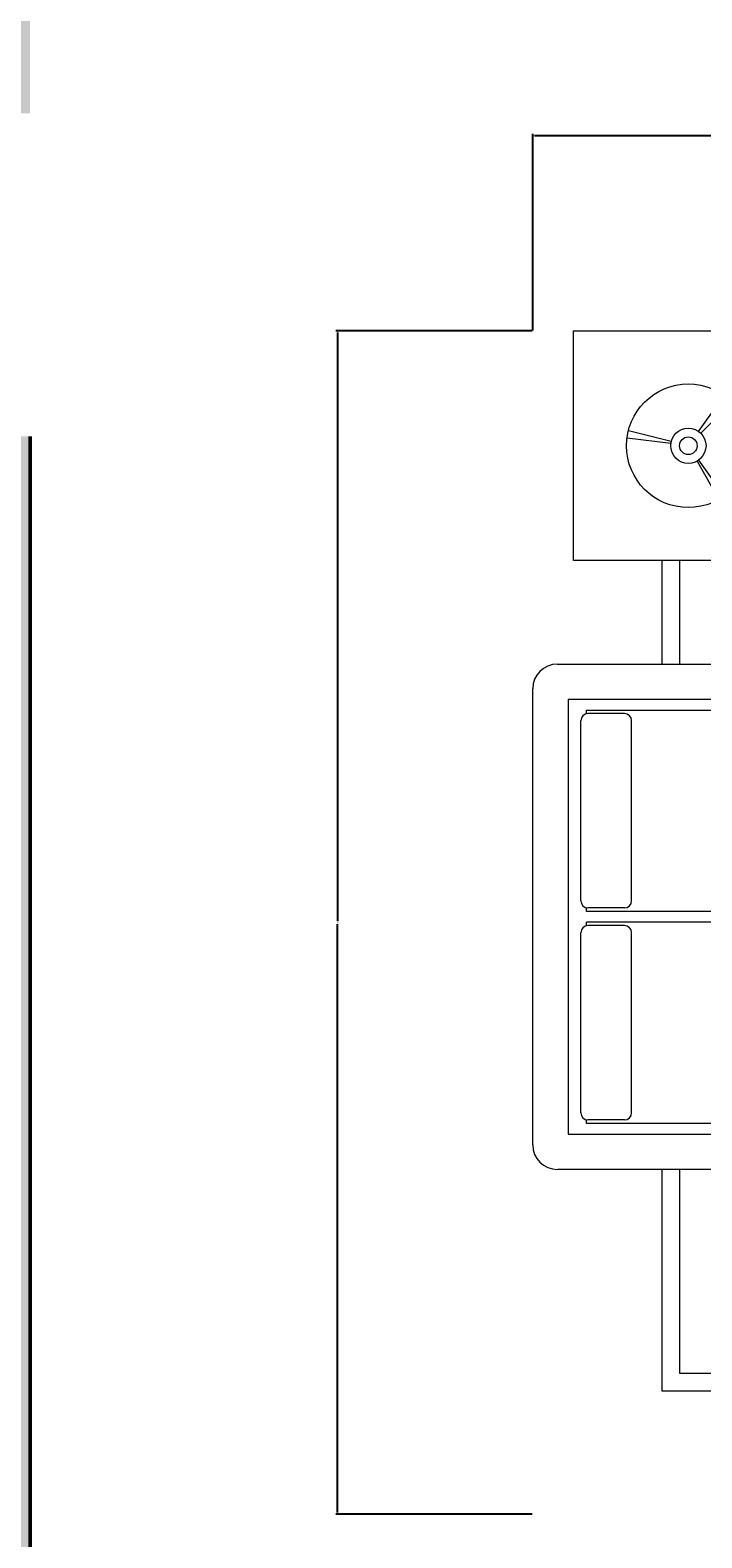
# Model space of a CAD drawing. Units: inches. Extents: x 2447 to 3157, y 2799 to 3988.
# Tile 5 of 9: x 2735 to 2810, y 3441 to 3609. Entities that reach past the tile are written whole.
import ezdxf

# ---------------------------------------------------------------- set-up
doc = ezdxf.new("R2010")
doc.units = ezdxf.units.IN
for name, color, linetype, lineweight in [('A-ANNO-DIMS', 2, 'Continuous', 18), ('A-FURN', 8, 'Continuous', 18), ('A-WALL', 7, 'Continuous', 50), ('A-WALL-PATT', 252, 'Continuous', 13)]:
    doc.layers.add(name, color=color, linetype=linetype, lineweight=lineweight)
doc.styles.get("Standard").update_dxf_attribs({"font": 'arial.ttf'})
doc.dimstyles.get("Standard").update_dxf_attribs({"dimtxt": 0.18, "dimasz": 0.18, "dimexe": 0.18, "dimexo": 0.0625, "dimgap": 0.09, "dimtad": 0, "dimtih": 1, "dimtoh": 1, "dimdec": 4, "dimzin": 0, "dimdsep": 46, "dimtxsty": 'Standard', "dimcen": 0.09, "dimadec": 0, "dimazin": 0, "dimtfac": 1, "dimtdec": 4, "dimtofl": 0, "dimtmove": 0, "dimatfit": 3, "dimfxl": 1, "dimtolj": 1, "dimtzin": 0, "dimarcsym": 0})

# ---------------------------------------------------------------- blocks, each defined once
blk = doc.blocks.new('A$C78064EA7')
for p, q in [((932.1, 3320.6), (2792.1, 3320.6)), ((862.1, 2740.6), (862.1, 3250.6)), ((2862.1, 3250.6), (2862.1, 2740.6)), ((962.1, 3220.6), (962.1, 2740.6)), ((2762.1, 3220.6), (962.1, 3220.6)), ((2762.1, 2740.6), (2762.1, 3220.6)), ((469.8, 3064.3), (542.4, 3166)), ((992.1, 3168.5), (1002.1, 3168.5)), ((992.1, 2570.6), (992.1, 3168.5)), ((1002.1, 3060.6), (1002.1, 3164.3)), ((1022.1, 3184.3), (1532.1, 3184.3)), ((1551.6, 3168.5), (1562.1, 3168.5)), ((1552.1, 3060.6), (1552.1, 3164.3)), ((1562.1, 2570.6), (1562.1, 3168.5)), ((1582.1, 3168.5), (1592.5, 3168.5)), ((1582.1, 2570.6), (1582.1, 3168.5)), ((1592.1, 3060.6), (1592.1, 3164.3)), ((1612.1, 3184.3), (2112.1, 3184.3)), ((2131.6, 3168.5), (2142.1, 3168.5)), ((2132.1, 3060.6), (2132.1, 3164.3)), ((2142.1, 2570.6), (2142.1, 3168.5)), ((2162.1, 3168.5), (2172.5, 3168.5)), ((2162.1, 2570.6), (2162.1, 3168.5)), ((2172.1, 3060.6), (2172.1, 3164.3)), ((2192.1, 3184.3), (2702.1, 3184.3)), ((2721.6, 3168.5), (2732.1, 3168.5)), ((2722.1, 3060.6), (2722.1, 3164.3)), ((2732.1, 3168.5), (2732.1, 2570.6)), ((3254.4, 3064.3), (3181.7, 3166)), ((476.1, 3059), (564.4, 3147.3)), ((3248.1, 3059), (3159.7, 3147.3)), ((391.1, 3029.8), (267.1, 3045.3)), ((392.2, 3035.7), (270.9, 3066)), ((1022.1, 3040.6), (1532.1, 3040.6)), ((1612.1, 3040.6), (2112.1, 3040.6)), ((2192.1, 3040.6), (2702.1, 3040.6)), ((3331.9, 3035.7), (3453.2, 3066)), ((3333, 3029.8), (3457.1, 3045.3)), ((465.5, 2980.2), (527.5, 2871.7)), ((469.8, 2982.9), (542.4, 2881.2)), ((3254.4, 2982.9), (3181.7, 2881.2)), ((3258.6, 2980.2), (3196.6, 2871.7)), ((862.1, 2823.6), (765.7, 2823.6)), ((2958.4, 2823.6), (2862.1, 2823.6)), ((862.1, 2773.6), (765.7, 2773.6)), ((2958.4, 2773.6), (2862.1, 2773.6)), ((962.1, 2760.6), (992.1, 2760.6)), ((2732.1, 2760.6), (2762.1, 2760.6)), ((365.7, 2698.6), (365.7, 2405.5)), ((415.7, 2698.6), (415.7, 2405.5)), ((942.1, 2720.6), (882.1, 2720.6)), ((2842.1, 2720.6), (2782.1, 2720.6)), ((3240.7, 2017.9), (3240.7, 2698.6)), ((3290.7, 2017.9), (3290.7, 2698.6)), ((992.1, 2623.6), (560, 2623.6)), ((560, 2405.5), (560, 2623.6)), ((992.1, 2573.6), (615.7, 2573.6)), ((615.7, 2573.6), (615.7, 2275.5)), ((1562.1, 2600.6), (1582.1, 2600.6)), ((2142.1, 2600.6), (2162.1, 2600.6)), ((1042.1, 2520.6), (1512.1, 2520.6)), ((1632.1, 2520.6), (2092.1, 2520.6)), ((2212.1, 2520.6), (2682.1, 2520.6)), ((70, 2405.5), (580, 2405.5)), ((600, 2385.5), (600, 2325.5)), ((0, 1045.5), (0, 2335.5)), ((580, 2305.5), (100, 2305.5)), ((100, 2305.5), (100, 1075.5)), ((560, 2275.5), (560, 2305.5)), ((152.1, 2275.5), (750, 2275.5)), ((152.1, 2265.1), (152.1, 2275.5)), ((260, 2265.5), (156.3, 2265.5)), ((136.3, 1735.5), (136.3, 2245.5)), ((280, 1735.5), (280, 2245.5)), ((800, 1755.5), (800, 2225.5)), ((3335.1, 2017.9), (3175.1, 2017.9)), ((3335.1, 1967.9), (3085.1, 1967.9)), ((3145.1, 1987.9), (3145.1, 1967.9)), ((3351.6, 1941.1), (3349.3, 1936.8)), ((3349.3, 1936.8), (3349.3, 1923.5)), ((3349.3, 1923.5), (3351.6, 1919.2)), ((3353.6, 1950), (3351.6, 1945.4)), ((3351.6, 1945.4), (3351.6, 1941.1)), ((3358.2, 1958.7), (3353.6, 1950)), ((3358.2, 1961), (3355.9, 1961)), ((3362.5, 1958.7), (3358.2, 1961)), ((3362.5, 1961), (3358.2, 1958.7)), ((3358.2, 1958.7), (3362.5, 1954.4)), ((3366.8, 1961), (3362.5, 1961)), ((3375.5, 1958.7), (3362.5, 1958.7)), ((3362.5, 1954.4), (3364.5, 1950)), ((3364.5, 1950), (3369.1, 1947.7)), ((3369.1, 1947.7), (3373.5, 1945.4)), ((3373.5, 1945.4), (3375.5, 1941.1)), ((3380.1, 1956.4), (3375.5, 1958.7)), ((3375.5, 1941.1), (3380.1, 1939.1)), ((3397.4, 1956.4), (3380.1, 1956.4)), ((3380.1, 1939.1), (3384.4, 1932.4)), ((3384.4, 1958.7), (3382.1, 1958.7)), ((3386.4, 1954.4), (3384.4, 1958.7)), ((3384.4, 1932.4), (3388.7, 1928.1)), ((3388.7, 1950), (3386.4, 1954.4)), ((3393.1, 1945.4), (3388.7, 1950)), ((3388.7, 1928.1), (3393.1, 1923.5)), ((3395.4, 1941.1), (3393.1, 1945.4)), ((3393.1, 1923.5), (3395.4, 1919.2)), ((3399.7, 1936.8), (3395.4, 1941.1)), ((3402, 1954.4), (3397.4, 1956.4)), ((3402, 1932.4), (3399.7, 1936.8)), ((3410.6, 1954.4), (3402, 1954.4)), ((3404, 1928.1), (3402, 1932.4)), ((3408.6, 1925.8), (3404, 1928.1)), ((3412.9, 1921.5), (3408.6, 1925.8)), ((3415, 1952.1), (3410.6, 1954.4)), ((3417.3, 1919.2), (3412.9, 1921.5)), ((3419.6, 1952.1), (3415, 1952.1)), ((3423.9, 1950), (3419.6, 1952.1)), ((3428.2, 1950), (3423.9, 1950)), ((3430.5, 1945.4), (3428.2, 1950)), ((3434.8, 1943.4), (3430.5, 1945.4)), ((3439.2, 1941.1), (3434.8, 1943.4)), ((3452.4, 1941.1), (3439.2, 1941.1)), ((3456.7, 1939.1), (3452.4, 1941.1)), ((3461.1, 1936.8), (3456.7, 1939.1)), ((3465.4, 1936.8), (3461.1, 1936.8)), ((3467.7, 1932.4), (3465.4, 1936.8)), ((3472, 1930.1), (3467.7, 1932.4)), ((3474.3, 1925.8), (3472, 1930.1)), ((3478.7, 1923.5), (3474.3, 1925.8)), ((3483, 1919.2), (3478.7, 1923.5)), ((3351.6, 1919.2), (3351.6, 1914.9)), ((3351.6, 1914.9), (3353.6, 1910.5)), ((3353.6, 1910.5), (3355.9, 1906.2)), ((3355.9, 1906.2), (3355.9, 1901.6)), ((3355.9, 1901.6), (3360.2, 1897.3)), ((3360.2, 1897.3), (3362.5, 1892.9)), ((3362.5, 1892.9), (3364.5, 1888.6)), ((3364.5, 1888.6), (3364.5, 1884.3)), ((3364.5, 1884.3), (3366.8, 1879.7)), ((3366.8, 1879.7), (3366.8, 1875.3)), ((3395.4, 1919.2), (3397.4, 1912.5)), ((3397.4, 1912.5), (3399.7, 1908.2)), ((3399.7, 1908.2), (3399.7, 1901.6)), ((3399.7, 1901.6), (3402, 1897.3)), ((3402, 1897.3), (3404, 1892.9)), ((3404, 1892.9), (3408.6, 1888.6)), ((3408.6, 1888.6), (3408.6, 1884.3)), ((3408.6, 1884.3), (3412.9, 1879.7)), ((3412.9, 1879.7), (3417.3, 1869)), ((3421.6, 1914.9), (3417.3, 1919.2)), ((3423.9, 1910.5), (3421.6, 1914.9)), ((3425.9, 1906.2), (3423.9, 1910.5)), ((3428.2, 1901.6), (3425.9, 1906.2)), ((3432.5, 1897.3), (3428.2, 1901.6)), ((3434.8, 1892.9), (3432.5, 1897.3)), ((3436.9, 1888.6), (3434.8, 1892.9)), ((3441.5, 1884.3), (3436.9, 1888.6)), ((3443.5, 1879.7), (3441.5, 1884.3)), ((3445.8, 1875.3), (3443.5, 1879.7)), ((3487.3, 1917.2), (3483, 1919.2)), ((3491.6, 1914.9), (3487.3, 1917.2)), ((3496.2, 1912.5), (3491.6, 1914.9)), ((3500.6, 1910.5), (3496.2, 1912.5)), ((3504.9, 1906.2), (3500.6, 1910.5)), ((3509.2, 1903.9), (3504.9, 1906.2)), ((3513.8, 1901.6), (3509.2, 1903.9)), ((3518.1, 1899.6), (3513.8, 1901.6)), ((3522.5, 1895.2), (3518.1, 1899.6)), ((3526.8, 1890.6), (3522.5, 1895.2)), ((3531.1, 1888.6), (3526.8, 1890.6)), ((3535.7, 1886.3), (3531.1, 1888.6)), ((3537.7, 1882), (3535.7, 1886.3)), ((3542.1, 1879.7), (3537.7, 1882)), ((3542.1, 1875.3), (3542.1, 1879.7)), ((2985.1, 1867.9), (2985.1, 1467.9)), ((3366.8, 1875.3), (3369.1, 1871)), ((3369.1, 1871), (3373.5, 1862.3)), ((3373.5, 1862.3), (3382.1, 1853.4)), ((3382.1, 1853.4), (3382.1, 1849.1)), ((3382.1, 1849.1), (3384.4, 1842.4)), ((3384.4, 1842.4), (3386.4, 1833.8)), ((3417.3, 1869), (3425.9, 1858)), ((3425.9, 1858), (3430.5, 1849.1)), ((3430.5, 1849.1), (3434.8, 1842.4)), ((3434.8, 1842.4), (3436.9, 1838.1)), ((3436.9, 1838.1), (3441.5, 1831.5)), ((3445.8, 1871), (3445.8, 1875.3)), ((3447.8, 1866.7), (3445.8, 1871)), ((3450.1, 1862.3), (3447.8, 1866.7)), ((3450.1, 1858), (3450.1, 1862.3)), ((3452.4, 1853.4), (3450.1, 1858)), ((3452.4, 1844.8), (3452.4, 1853.4)), ((3454.4, 1838.1), (3452.4, 1844.8)), ((3454.4, 1833.8), (3454.4, 1838.1)), ((3546.7, 1873.3), (3542.1, 1875.3)), ((3548.7, 1869), (3546.7, 1873.3)), ((3551, 1864.4), (3548.7, 1869)), ((3555.3, 1860), (3551, 1864.4)), ((3557.6, 1855.7), (3555.3, 1860)), ((3561.9, 1853.4), (3557.6, 1855.7)), ((3561.9, 1849.1), (3561.9, 1853.4)), ((3566.3, 1847.1), (3561.9, 1849.1)), ((3568.6, 1842.4), (3566.3, 1847.1)), ((3570.6, 1838.1), (3568.6, 1842.4)), ((3574.9, 1836.1), (3570.6, 1838.1)), ((3574.9, 1831.5), (3574.9, 1836.1)), ((3386.4, 1833.8), (3391, 1825.1)), ((3391, 1825.1), (3391, 1820.5)), ((3391, 1820.5), (3393.1, 1811.9)), ((3393.1, 1811.9), (3393.1, 1805.2)), ((3393.1, 1805.2), (3395.4, 1798.6)), ((3395.4, 1798.6), (3395.4, 1792.2)), ((3395.4, 1792.2), (3399.7, 1783.3)), ((3441.5, 1831.5), (3443.5, 1825.1)), ((3443.5, 1825.1), (3445.8, 1820.5)), ((3445.8, 1820.5), (3445.8, 1816.2)), ((3445.8, 1816.2), (3447.8, 1809.6)), ((3447.8, 1809.6), (3447.8, 1805.2)), ((3447.8, 1805.2), (3450.1, 1798.6)), ((3450.1, 1798.6), (3452.4, 1794.3)), ((3452.4, 1794.3), (3452.4, 1774.7)), ((3456.7, 1829.5), (3454.4, 1833.8)), ((3458.8, 1825.1), (3456.7, 1829.5)), ((3461.1, 1820.5), (3458.8, 1825.1)), ((3463.4, 1816.2), (3461.1, 1820.5)), ((3463.4, 1811.9), (3463.4, 1816.2)), ((3465.4, 1805.2), (3463.4, 1811.9)), ((3465.4, 1798.6), (3465.4, 1805.2)), ((3467.7, 1794.3), (3465.4, 1798.6)), ((3467.7, 1789.9), (3467.7, 1794.3)), ((3579.5, 1831.5), (3574.9, 1831.5)), ((3581.5, 1827.2), (3579.5, 1831.5)), ((3585.9, 1825.1), (3581.5, 1827.2)), ((3585.9, 1820.5), (3585.9, 1825.1)), ((3590.5, 1816.2), (3585.9, 1820.5)), ((3592.5, 1811.9), (3590.5, 1816.2)), ((3594.8, 1807.5), (3592.5, 1811.9)), ((3596.8, 1803.2), (3594.8, 1807.5)), ((3599.1, 1798.6), (3596.8, 1803.2)), ((3601.4, 1794.3), (3599.1, 1798.6)), ((3605.7, 1792.2), (3601.4, 1794.3)), ((3610.1, 1787.6), (3605.7, 1792.2)), ((3399.7, 1783.3), (3399.7, 1763.7)), ((3399.7, 1763.7), (3408.6, 1746.1)), ((3452.4, 1774.7), (3454.4, 1768)), ((3454.4, 1768), (3456.7, 1761.4)), ((3456.7, 1761.4), (3458.8, 1755)), ((3458.8, 1755), (3461.1, 1750.4)), ((3461.1, 1750.4), (3463.4, 1746.1)), ((3472, 1783.3), (3467.7, 1789.9)), ((3474.3, 1779), (3472, 1783.3)), ((3474.3, 1774.7), (3474.3, 1779)), ((3476.3, 1770.3), (3474.3, 1774.7)), ((3476.3, 1761.4), (3476.3, 1770.3)), ((3478.7, 1757.1), (3476.3, 1761.4)), ((3478.7, 1733.1), (3478.7, 1757.1)), ((3612.4, 1783.3), (3610.1, 1787.6)), ((3614.4, 1779), (3612.4, 1783.3)), ((3616.7, 1774.7), (3614.4, 1779)), ((3616.7, 1766), (3616.7, 1774.7)), ((3618.7, 1761.4), (3616.7, 1766)), ((3618.7, 1757.1), (3618.7, 1761.4)), ((3621, 1752.7), (3618.7, 1757.1)), ((3621, 1748.4), (3621, 1752.7)), ((152.1, 1705.5), (152.1, 1716)), ((260, 1715.5), (156.3, 1715.5)), ((3408.6, 1746.1), (3408.6, 1717.5)), ((3408.6, 1717.5), (3417.3, 1708.9)), ((3417.3, 1708.9), (3417.3, 1691.3)), ((3463.4, 1746.1), (3465.4, 1739.5)), ((3465.4, 1739.5), (3467.7, 1735.1)), ((3467.7, 1735.1), (3469.7, 1730.8)), ((3469.7, 1730.8), (3469.7, 1700.2)), ((3480.7, 1728.5), (3478.7, 1733.1)), ((3480.7, 1708.9), (3480.7, 1728.5)), ((3483, 1704.6), (3480.7, 1708.9)), ((3623.3, 1744.1), (3621, 1748.4)), ((3625.3, 1739.5), (3623.3, 1744.1)), ((3627.6, 1735.1), (3625.3, 1739.5)), ((3625.3, 1722.1), (3627.6, 1726.5)), ((3625.3, 1704.6), (3625.3, 1722.1)), ((3627.6, 1726.5), (3627.6, 1735.1)), ((750, 1705.5), (152.1, 1705.5)), ((750, 1675.5), (152.1, 1675.5)), ((152.1, 1665.1), (152.1, 1675.5)), ((260, 1665.5), (156.3, 1665.5)), ((720, 1685.5), (720, 1705.5)), ((720, 1675.5), (720, 1695.5)), ((3417.3, 1691.3), (3425.9, 1674)), ((3425.9, 1674), (3425.9, 1656.4)), ((3469.7, 1700.2), (3478.7, 1682.6)), ((3478.7, 1682.6), (3478.7, 1656.4)), ((3483, 1700.2), (3483, 1704.6)), ((3485.3, 1695.6), (3483, 1700.2)), ((3487.3, 1691.3), (3485.3, 1695.6)), ((3491.6, 1678.3), (3487.3, 1691.3)), ((3493.9, 1669.4), (3491.6, 1678.3)), ((3496.2, 1665), (3493.9, 1669.4)), ((3496.2, 1660.7), (3496.2, 1665)), ((3627.6, 1700.2), (3625.3, 1704.6)), ((3627.6, 1691.3), (3627.6, 1700.2)), ((3629.9, 1687), (3627.6, 1691.3)), ((3629.9, 1669.4), (3629.9, 1687)), ((3632, 1665), (3629.9, 1669.4)), ((3632, 1656.4), (3632, 1665)), ((136.3, 1135.5), (136.3, 1645.5)), ((280, 1135.5), (280, 1645.5)), ((800, 1155.5), (800, 1625.5)), ((3425.9, 1656.4), (3434.8, 1638.8)), ((3434.8, 1638.8), (3434.8, 1634.5)), ((3434.8, 1634.5), (3436.9, 1630.1)), ((3436.9, 1630.1), (3436.9, 1571)), ((3478.7, 1656.4), (3487.3, 1647.4)), ((3487.3, 1647.4), (3487.3, 1636.5)), ((3487.3, 1636.5), (3489.6, 1632.1)), ((3489.6, 1632.1), (3489.6, 1627.8)), ((3489.6, 1627.8), (3491.6, 1623.5)), ((3491.6, 1623.5), (3491.6, 1538.1)), ((3498.2, 1656.4), (3496.2, 1660.7)), ((3498.2, 1645.4), (3498.2, 1656.4)), ((3500.6, 1641.1), (3498.2, 1645.4)), ((3500.6, 1627.8), (3500.6, 1641.1)), ((3502.6, 1621.2), (3500.6, 1627.8)), ((3627.6, 1621.2), (3629.9, 1625.5)), ((3629.9, 1652), (3632, 1656.4)), ((3629.9, 1625.5), (3629.9, 1652)), ((3504.9, 1614.5), (3502.6, 1621.2)), ((3504.9, 1605.9), (3504.9, 1614.5)), ((3507.2, 1599.3), (3504.9, 1605.9)), ((3507.2, 1586.3), (3507.2, 1599.3)), ((3509.2, 1579.6), (3507.2, 1586.3)), ((3509.2, 1575.3), (3509.2, 1579.6)), ((3614.4, 1575.3), (3616.7, 1582)), ((3616.7, 1586.3), (3618.7, 1590.6)), ((3616.7, 1582), (3616.7, 1586.3)), ((3618.7, 1594.9), (3621, 1599.3)), ((3618.7, 1590.6), (3618.7, 1594.9)), ((3621, 1599.3), (3623.3, 1603.9)), ((3623.3, 1603.9), (3625.3, 1608.2)), ((3625.3, 1612.5), (3627.6, 1616.9)), ((3625.3, 1608.2), (3625.3, 1612.5)), ((3627.6, 1616.9), (3627.6, 1621.2)), ((3436.9, 1571), (3439.2, 1564.4)), ((3439.2, 1564.4), (3439.2, 1527.1)), ((3491.6, 1538.1), (3489.6, 1529.2)), ((3504.9, 1557.7), (3507.2, 1562)), ((3504.9, 1518.2), (3504.9, 1557.7)), ((3507.2, 1571), (3509.2, 1575.3)), ((3507.2, 1562), (3507.2, 1571)), ((3596.8, 1533.5), (3599.1, 1538.1)), ((3599.1, 1538.1), (3601.4, 1542.4)), ((3601.4, 1542.4), (3603.4, 1549.1)), ((3603.4, 1549.1), (3605.7, 1553.4)), ((3605.7, 1553.4), (3607.8, 1557.7)), ((3607.8, 1562), (3610.1, 1566.4)), ((3607.8, 1557.7), (3607.8, 1562)), ((3610.1, 1566.4), (3612.4, 1571)), ((3612.4, 1571), (3614.4, 1575.3)), ((3439.2, 1527.1), (3436.9, 1522.5)), ((3436.9, 1522.5), (3436.9, 1505.2)), ((3436.9, 1505.2), (3439.2, 1500.9)), ((3439.2, 1500.9), (3441.5, 1496.3)), ((3441.5, 1496.3), (3441.5, 1491.9)), ((3487.3, 1507.2), (3485.3, 1496.3)), ((3485.3, 1496.3), (3485.3, 1479)), ((3489.6, 1516.2), (3487.3, 1511.9)), ((3487.3, 1511.9), (3487.3, 1507.2)), ((3489.6, 1529.2), (3489.6, 1516.2)), ((3500.6, 1502.9), (3502.6, 1509.5)), ((3500.6, 1476.7), (3500.6, 1502.9)), ((3502.6, 1513.9), (3504.9, 1518.2)), ((3502.6, 1509.5), (3502.6, 1513.9)), ((3551, 1489.9), (3564, 1502.9)), ((3564, 1502.9), (3572.9, 1509.5)), ((3572.9, 1509.5), (3577.2, 1513.9)), ((3577.2, 1513.9), (3581.5, 1516.2)), ((3581.5, 1516.2), (3583.8, 1520.5)), ((3583.8, 1520.5), (3588.2, 1522.5)), ((3588.2, 1522.5), (3590.5, 1527.1)), ((3590.5, 1527.1), (3594.8, 1529.2)), ((3594.8, 1529.2), (3596.8, 1533.5)), ((3441.5, 1491.9), (3443.5, 1487.6)), ((3443.5, 1487.6), (3443.5, 1461.4)), ((3443.5, 1461.4), (3445.8, 1457)), ((3445.8, 1457), (3445.8, 1448.1)), ((3485.3, 1479), (3483, 1472.3)), ((3483, 1472.3), (3483, 1450.4)), ((3493.9, 1450.4), (3496.2, 1454.7)), ((3496.2, 1463.4), (3498.2, 1468)), ((3496.2, 1454.7), (3496.2, 1463.4)), ((3498.2, 1472.3), (3500.6, 1476.7)), ((3498.2, 1468), (3498.2, 1472.3)), ((3531.1, 1454.7), (3533.4, 1461.4)), ((3531.1, 1450.4), (3531.1, 1454.7)), ((3533.4, 1461.4), (3535.7, 1465.7)), ((3535.7, 1465.7), (3537.7, 1470)), ((3537.7, 1470), (3540, 1474.3)), ((3540, 1474.3), (3542.1, 1479)), ((3542.1, 1479), (3544.4, 1483.3)), ((3544.4, 1483.3), (3548.7, 1485.3)), ((3548.7, 1485.3), (3551, 1489.9)), ((3445.8, 1448.1), (3447.8, 1443.8)), ((3447.8, 1443.8), (3447.8, 1439.4)), ((3447.8, 1439.4), (3450.1, 1435.1)), ((3450.1, 1435.1), (3450.1, 1426.2)), ((3450.1, 1426.2), (3452.4, 1421.8)), ((3452.4, 1421.8), (3456.7, 1417.5)), ((3456.7, 1417.5), (3458.8, 1413.2)), ((3458.8, 1413.2), (3472, 1413.2)), ((3474.3, 1419.8), (3472, 1415.2)), ((3472, 1415.2), (3472, 1413.2)), ((3472, 1413.2), (3476.3, 1410.9)), ((3476.3, 1424.2), (3474.3, 1419.8)), ((3478.7, 1428.5), (3476.3, 1424.2)), ((3476.3, 1410.9), (3480.7, 1413.2)), ((3480.7, 1437.1), (3478.7, 1432.8)), ((3478.7, 1432.8), (3478.7, 1428.5)), ((3483, 1450.4), (3480.7, 1446.1)), ((3480.7, 1446.1), (3480.7, 1437.1)), ((3480.7, 1413.2), (3485.3, 1415.2)), ((3485.3, 1417.5), (3487.3, 1421.8)), ((3485.3, 1413.2), (3485.3, 1417.5)), ((3485.3, 1415.2), (3489.6, 1417.5)), ((3487.3, 1421.8), (3489.6, 1426.2)), ((3489.6, 1435.1), (3491.6, 1439.4)), ((3489.6, 1426.2), (3489.6, 1435.1)), ((3489.6, 1417.5), (3496.2, 1421.8)), ((3491.6, 1439.4), (3493.9, 1443.8)), ((3493.9, 1443.8), (3493.9, 1450.4)), ((3496.2, 1421.8), (3500.6, 1424.2)), ((3500.6, 1424.2), (3504.9, 1426.2)), ((3504.9, 1426.2), (3509.2, 1426.2)), ((3509.2, 1426.2), (3511.5, 1430.5)), ((3511.5, 1430.5), (3515.8, 1430.5)), ((3515.8, 1430.5), (3518.1, 1435.1)), ((3518.1, 1435.1), (3522.5, 1439.4)), ((3522.5, 1439.4), (3524.8, 1443.8)), ((3524.8, 1443.8), (3529.1, 1446.1)), ((3529.1, 1446.1), (3531.1, 1450.4)), ((3335.1, 1367.9), (3085.1, 1367.9)), ((3145.1, 1367.9), (3145.1, 1347.9)), ((3175.1, 1317.9), (3335.1, 1317.9)), ((152.1, 1105.5), (152.1, 1115.5)), ((260, 1115.5), (156.3, 1115.5)), ((100, 1075.5), (580, 1075.5)), ((750, 1105.5), (152.1, 1105.5)), ((560, 1075.5), (560, 1105.5)), ((600, 1055.5), (600, 995.5)), ((580, 975.5), (70, 975.5)), ((2261.5, 700), (1861.5, 700)), ((1761.5, 350), (1761.5, 600)), ((2361.5, 350), (2361.5, 600)), ((1761.5, 540), (1741.5, 540)), ((2381.5, 540), (2361.5, 540)), ((1711.5, 510), (1711.5, 350)), ((2411.5, 350), (2411.5, 510)), ((2236.1, 300.7), (2227.4, 298.6)), ((2242.7, 303), (2236.1, 300.7)), ((2247, 303), (2242.7, 303)), ((2256, 311.6), (2247, 303)), ((2264.6, 315.9), (2256, 311.6)), ((2269, 318.2), (2264.6, 315.9)), ((2273.3, 318.2), (2269, 318.2)), ((2277.9, 320.5), (2273.3, 318.2)), ((2282.2, 320.5), (2277.9, 320.5)), ((2286.6, 322.6), (2282.2, 320.5)), ((2290.9, 324.9), (2286.6, 322.6)), ((2295.2, 329.2), (2290.9, 324.9)), ((2299.8, 329.2), (2295.2, 329.2)), ((2304.2, 331.5), (2299.8, 329.2)), ((2308.5, 333.5), (2304.2, 331.5)), ((2312.8, 333.5), (2308.5, 333.5)), ((2317.1, 335.8), (2312.8, 333.5)), ((2330.4, 335.8), (2317.1, 335.8)), ((2326.1, 300.7), (2321.8, 296.3)), ((2332.7, 305), (2326.1, 300.7)), ((2334.7, 333.5), (2330.4, 335.8)), ((2334.7, 309.6), (2332.7, 305)), ((2339.1, 333.5), (2334.7, 333.5)), ((2339.1, 311.6), (2334.7, 309.6)), ((2343.7, 331.5), (2339.1, 333.5)), ((2341.4, 315.9), (2339.1, 311.6)), ((2343.7, 320.5), (2341.4, 315.9)), ((2352.3, 326.9), (2343.7, 331.5)), ((2348, 322.6), (2343.7, 320.5)), ((2352.3, 326.9), (2348, 322.6)), ((2348, 298.6), (2352.3, 300.7)), ((2350, 305), (2352.3, 309.6)), ((2350, 287.7), (2350, 305)), ((2352.3, 322.6), (2354.6, 326.9)), ((2354.6, 322.6), (2352.3, 326.9)), ((2352.3, 309.6), (2352.3, 322.6)), ((2352.3, 300.7), (2352.3, 303)), ((2354.6, 326.9), (2354.6, 329.2)), ((2354.6, 318.2), (2354.6, 322.6)), ((2050, 259.2), (2032.4, 250.2)), ((2067.6, 259.2), (2050, 259.2)), ((2084.9, 267.8), (2067.6, 259.2)), ((2102.5, 267.8), (2084.9, 267.8)), ((2111.2, 276.5), (2102.5, 267.8)), ((2139.7, 276.5), (2111.2, 276.5)), ((2157.3, 285.4), (2139.7, 276.5)), ((2176.9, 285.4), (2157.3, 285.4)), ((2185.9, 289.7), (2176.9, 285.4)), ((2192.2, 289.7), (2185.9, 289.7)), ((2198.9, 292), (2192.2, 289.7)), ((2205.5, 292), (2198.9, 292)), ((2214.2, 294), (2205.5, 292)), ((2218.8, 294), (2214.2, 294)), ((2227.4, 298.6), (2218.8, 294)), ((2251.7, 259.2), (2242.7, 254.6)), ((2262.6, 267.8), (2251.7, 259.2)), ((2273.3, 272.1), (2262.6, 267.8)), ((2277.9, 276.5), (2273.3, 272.1)), ((2282.2, 276.5), (2277.9, 276.5)), ((2286.6, 281.1), (2282.2, 276.5)), ((2290.9, 283.1), (2286.6, 281.1)), ((2295.2, 285.4), (2290.9, 283.1)), ((2290.9, 252.5), (2295.2, 256.9)), ((2301.9, 285.4), (2295.2, 285.4)), ((2295.2, 256.9), (2299.8, 259.2)), ((2299.8, 259.2), (2304.2, 261.2)), ((2306.2, 287.7), (2301.9, 285.4)), ((2304.2, 261.2), (2308.5, 263.5)), ((2312.8, 289.7), (2306.2, 287.7)), ((2308.5, 263.5), (2312.8, 267.8)), ((2317.1, 292), (2312.8, 289.7)), ((2312.8, 267.8), (2315.1, 272.1)), ((2315.1, 272.1), (2319.5, 276.5)), ((2321.8, 296.3), (2317.1, 292)), ((2319.5, 276.5), (2321.8, 281.1)), ((2321.8, 281.1), (2326.1, 283.1)), ((2326.1, 283.1), (2330.4, 285.4)), ((2330.4, 285.4), (2334.7, 289.7)), ((2334.7, 289.7), (2339.1, 292)), ((2339.1, 292), (2343.7, 296.3)), ((2339.1, 254.6), (2343.7, 256.9)), ((2343.7, 296.3), (2348, 298.6)), ((2343.7, 261.2), (2345.7, 265.5)), ((2343.7, 256.9), (2343.7, 261.2)), ((2345.7, 270.1), (2348, 274.4)), ((2345.7, 265.5), (2345.7, 270.1)), ((2348, 283.1), (2350, 287.7)), ((2348, 274.4), (2348, 283.1)), ((1811.2, 228.3), (1806.8, 226.3)), ((1806.8, 226.3), (1806.8, 213.1)), ((1815.5, 232.7), (1811.2, 228.3)), ((1819.8, 235), (1815.5, 232.7)), ((1828.8, 235), (1819.8, 235)), ((1833.1, 237.3), (1828.8, 235)), ((1837.4, 237.3), (1833.1, 237.3)), ((1841.7, 239.3), (1837.4, 237.3)), ((1850.7, 239.3), (1841.7, 239.3)), ((1855, 241.6), (1850.7, 239.3)), ((1881.3, 241.6), (1855, 241.6)), ((1885.6, 243.6), (1881.3, 241.6)), ((1889.9, 243.6), (1885.6, 243.6)), ((1894.5, 245.9), (1889.9, 243.6)), ((1898.9, 248.2), (1894.5, 245.9)), ((1916.2, 248.2), (1898.9, 248.2)), ((1920.8, 245.9), (1916.2, 248.2)), ((1958, 245.9), (1920.8, 245.9)), ((1964.6, 248.2), (1958, 245.9)), ((2023.8, 248.2), (1964.6, 248.2)), ((2028.1, 250.2), (2023.8, 248.2)), ((2032.4, 250.2), (2028.1, 250.2)), ((2093.9, 215.4), (2076.3, 206.4)), ((2124.4, 215.4), (2093.9, 215.4)), ((2128.8, 217.4), (2124.4, 215.4)), ((2133.1, 219.7), (2128.8, 217.4)), ((2139.7, 221.7), (2133.1, 219.7)), ((2144.1, 224), (2139.7, 221.7)), ((2148.7, 226.3), (2144.1, 224)), ((2155, 228.3), (2148.7, 226.3)), ((2161.7, 230.6), (2155, 228.3)), ((2168.3, 232.7), (2161.7, 230.6)), ((2187.9, 232.7), (2168.3, 232.7)), ((2176.9, 213.1), (2183.6, 217.4)), ((2183.6, 217.4), (2187.9, 217.4)), ((2192.2, 235), (2187.9, 232.7)), ((2187.9, 217.4), (2192.2, 219.7)), ((2198.9, 237.3), (2192.2, 235)), ((2192.2, 219.7), (2198.9, 219.7)), ((2203.2, 237.3), (2198.9, 237.3)), ((2198.9, 219.7), (2205.5, 221.7)), ((2209.8, 239.3), (2203.2, 237.3)), ((2205.5, 221.7), (2209.8, 221.7)), ((2214.2, 239.3), (2209.8, 239.3)), ((2209.8, 221.7), (2214.2, 224)), ((2218.8, 241.6), (2214.2, 239.3)), ((2214.2, 224), (2218.8, 226.3)), ((2225.1, 243.6), (2218.8, 241.6)), ((2218.8, 226.3), (2223.1, 228.3)), ((2223.1, 228.3), (2227.4, 230.6)), ((2231.8, 248.2), (2225.1, 243.6)), ((2227.4, 230.6), (2231.8, 230.6)), ((2236.1, 250.2), (2231.8, 248.2)), ((2231.8, 230.6), (2238.4, 232.7)), ((2242.7, 254.6), (2236.1, 250.2)), ((2238.4, 232.7), (2247, 232.7)), ((2247, 232.7), (2251.7, 235)), ((2251.7, 235), (2256, 235)), ((2256, 235), (2260.3, 237.3)), ((2260.3, 237.3), (2264.6, 239.3)), ((2264.6, 239.3), (2269, 239.3)), ((2269, 239.3), (2273.3, 241.6)), ((2273.3, 241.6), (2277.9, 243.6)), ((2277.9, 243.6), (2282.2, 248.2)), ((2282.2, 248.2), (2286.6, 250.2)), ((2286.6, 250.2), (2290.9, 252.5)), ((2323.8, 213.1), (2326.1, 217.4)), ((2326.1, 217.4), (2330.4, 219.7)), ((2330.4, 224), (2332.7, 228.3)), ((2330.4, 219.7), (2330.4, 224)), ((2332.7, 228.3), (2334.7, 232.7)), ((2334.7, 245.9), (2337.1, 250.2)), ((2334.7, 232.7), (2334.7, 245.9)), ((2337.1, 250.2), (2339.1, 254.6)), ((1806.8, 213.1), (1804.5, 208.7)), ((1804.5, 208.7), (1806.8, 204.4)), ((1808.9, 213.1), (1806.8, 213.1)), ((1806.8, 204.4), (1808.9, 199.8)), ((1806.8, 199.8), (1811.2, 199.8)), ((1813.5, 210.7), (1808.9, 213.1)), ((1808.9, 199.8), (1811.2, 195.5)), ((1811.2, 199.8), (1815.5, 197.8)), ((1811.2, 195.5), (1815.5, 188.8)), ((1817.8, 208.7), (1813.5, 210.7)), ((1815.5, 197.8), (1819.8, 195.5)), ((1815.5, 188.8), (1817.8, 184.5)), ((1822.1, 206.4), (1817.8, 208.7)), ((1817.8, 184.5), (1819.8, 180.2)), ((1819.8, 195.5), (1828.8, 195.5)), ((1819.8, 180.2), (1819.8, 175.9)), ((1819.8, 175.9), (1824.1, 173.6)), ((1826.5, 206.4), (1822.1, 206.4)), ((1824.1, 173.6), (1824.1, 169.2)), ((1830.8, 204.4), (1826.5, 206.4)), ((1828.8, 195.5), (1833.1, 193.5)), ((1839.7, 204.4), (1830.8, 204.4)), ((1833.1, 193.5), (1837.4, 191.2)), ((1837.4, 191.2), (1844, 191.2)), ((1844, 202.1), (1839.7, 204.4)), ((1866, 202.1), (1844, 202.1)), ((1844, 191.2), (1848.4, 188.8)), ((1848.4, 188.8), (1857, 188.8)), ((1857, 188.8), (1861.6, 186.8)), ((1861.6, 186.8), (1866, 186.8)), ((1872.6, 199.8), (1866, 202.1)), ((1866, 186.8), (1870.3, 184.5)), ((1870.3, 184.5), (1896.6, 184.5)), ((1889.9, 199.8), (1872.6, 199.8)), ((1900.9, 197.8), (1889.9, 199.8)), ((1896.6, 184.5), (1903.2, 182.5)), ((1905.5, 197.8), (1900.9, 197.8)), ((1903.2, 182.5), (1907.5, 182.5)), ((1909.8, 195.5), (1905.5, 197.8)), ((1907.5, 182.5), (1911.8, 180.2)), ((1922.8, 195.5), (1909.8, 195.5)), ((1911.8, 180.2), (1951.4, 180.2)), ((1931.7, 193.5), (1922.8, 195.5)), ((2017.1, 193.5), (1931.7, 193.5)), ((1951.4, 180.2), (1955.7, 177.9)), ((1955.7, 177.9), (1964.6, 177.9)), ((1964.6, 177.9), (1969, 175.9)), ((1969, 175.9), (1973.3, 175.9)), ((1973.3, 175.9), (1979.9, 177.9)), ((1979.9, 177.9), (1992.9, 177.9)), ((1992.9, 177.9), (1999.5, 180.2)), ((1999.5, 180.2), (2008.2, 180.2)), ((2008.2, 180.2), (2014.8, 182.5)), ((2014.8, 182.5), (2021.5, 184.5)), ((2021.5, 195.5), (2017.1, 193.5)), ((2025.8, 195.5), (2021.5, 195.5)), ((2021.5, 184.5), (2034.7, 184.5)), ((2030.1, 197.8), (2025.8, 195.5)), ((2041.1, 197.8), (2030.1, 197.8)), ((2034.7, 184.5), (2039.1, 186.8)), ((2039.1, 186.8), (2050, 186.8)), ((2050, 206.4), (2041.1, 197.8)), ((2076.3, 206.4), (2050, 206.4)), ((2050, 186.8), (2054.3, 188.8)), ((2054.3, 188.8), (2058.7, 188.8)), ((2058.7, 188.8), (2063, 191.2)), ((2063, 191.2), (2071.9, 193.5)), ((2071.9, 193.5), (2084.9, 197.8)), ((2084.9, 197.8), (2089.3, 199.8)), ((2089.3, 199.8), (2093.9, 202.1)), ((2093.9, 202.1), (2098.2, 202.1)), ((2098.2, 202.1), (2102.5, 204.4)), ((2102.5, 204.4), (2122.1, 204.4)), ((2122.1, 204.4), (2126.8, 206.4)), ((2126.8, 206.4), (2150.7, 206.4)), ((2150.7, 206.4), (2155, 208.7)), ((2155, 208.7), (2164, 208.7)), ((2164, 208.7), (2168.3, 210.7)), ((2168.3, 210.7), (2172.6, 210.7)), ((2172.6, 210.7), (2176.9, 213.1)), ((2293.2, 166.9), (2295.2, 171.3)), ((2295.2, 171.3), (2297.5, 175.9)), ((2297.5, 175.9), (2299.8, 180.2)), ((2299.8, 180.2), (2304.2, 184.5)), ((2304.2, 184.5), (2306.2, 188.8)), ((2306.2, 188.8), (2308.5, 193.5)), ((2308.5, 193.5), (2310.8, 197.8)), ((2310.8, 197.8), (2312.8, 202.1)), ((2312.8, 202.1), (2317.1, 206.4)), ((2317.1, 206.4), (2319.5, 210.7)), ((2319.5, 210.7), (2323.8, 213.1)), ((1824.1, 169.2), (1828.8, 166.9)), ((1828.8, 166.9), (1833.1, 162.6)), ((1833.1, 162.6), (1837.4, 160.3)), ((1837.4, 160.3), (1839.7, 156)), ((1839.7, 156), (1844, 154)), ((1844, 154), (1848.4, 154)), ((1848.4, 154), (1855, 151.7)), ((1855, 151.7), (1859.3, 149.4)), ((1859.3, 149.4), (1863.7, 147.3)), ((1863.7, 147.3), (1868, 145)), ((1868, 145), (1872.6, 143)), ((1872.6, 143), (1876.9, 140.7)), ((1876.9, 140.7), (1879, 136.4)), ((1879, 136.4), (1883.6, 134.1)), ((1883.6, 134.1), (1896.6, 121.1)), ((2249.4, 127.5), (2253.7, 129.8)), ((2253.7, 129.8), (2258, 134.1)), ((2258, 134.1), (2262.6, 136.4)), ((2262.6, 136.4), (2267, 138.4)), ((2267, 138.4), (2269, 143)), ((2269, 143), (2273.3, 143)), ((2273.3, 143), (2275.6, 147.3)), ((2275.6, 147.3), (2279.9, 149.4)), ((2279.9, 149.4), (2282.2, 154)), ((2282.2, 154), (2284.3, 158.3)), ((2284.3, 158.3), (2288.9, 162.6)), ((2288.9, 162.6), (2293.2, 166.9)), ((1896.6, 121.1), (1903.2, 112.2)), ((1903.2, 112.2), (1907.5, 107.9)), ((1907.5, 107.9), (1909.8, 103.5)), ((1909.8, 103.5), (1914.1, 101.2)), ((1914.1, 101.2), (1916.2, 96.9)), ((1916.2, 96.9), (1920.8, 94.6)), ((1920.8, 94.6), (1922.8, 90.3)), ((1922.8, 90.3), (1927.1, 88.3)), ((1927.1, 88.3), (1931.7, 86)), ((1931.7, 86), (1936.1, 83.7)), ((2187.9, 83.7), (2192.2, 86)), ((2192.2, 86), (2196.9, 88.3)), ((2196.9, 88.3), (2201.2, 90.3)), ((2201.2, 90.3), (2205.5, 92.6)), ((2205.5, 92.6), (2209.8, 94.6)), ((2209.8, 94.6), (2214.2, 99.2)), ((2214.2, 99.2), (2218.8, 99.2)), ((2218.8, 99.2), (2220.8, 103.5)), ((2220.8, 103.5), (2225.1, 105.6)), ((2225.1, 110.2), (2229.7, 110.2)), ((2225.1, 105.6), (2225.1, 110.2)), ((2229.7, 110.2), (2231.8, 114.5)), ((2231.8, 114.5), (2236.1, 116.5)), ((2236.1, 116.5), (2240.7, 118.8)), ((2240.7, 118.8), (2242.7, 123.1)), ((2242.7, 123.1), (2247, 123.1)), ((2247, 123.1), (2249.4, 127.5)), ((1936.1, 83.7), (1942.7, 81.6)), ((1942.7, 81.6), (1947, 79.3)), ((1947, 79.3), (1951.4, 77.3)), ((1951.4, 77.3), (1955.7, 77.3)), ((1955.7, 77.3), (1960, 75)), ((1960, 75), (1964.6, 72.7)), ((1964.6, 72.7), (1969, 70.7)), ((1969, 70.7), (1975.6, 68.4)), ((1975.6, 68.4), (1979.9, 68.4)), ((1979.9, 68.4), (1984.2, 66.4)), ((1984.2, 66.4), (1988.6, 66.4)), ((1988.6, 66.4), (1992.9, 64.1)), ((1992.9, 64.1), (1997.5, 61.8)), ((1997.5, 61.8), (2001.8, 59.7)), ((2001.8, 59.7), (2006.2, 59.7)), ((2006.2, 59.7), (2010.5, 57.4)), ((2010.5, 57.4), (2014.8, 57.4)), ((2014.8, 57.4), (2019.2, 55.1)), ((2019.2, 55.1), (2045.7, 55.1)), ((2045.7, 55.1), (2050, 53.1)), ((2050, 53.1), (2058.7, 53.1)), ((2058.7, 53.1), (2063, 55.1)), ((2063, 55.1), (2080.6, 55.1)), ((2080.6, 55.1), (2084.9, 57.4)), ((2084.9, 57.4), (2093.9, 57.4)), ((2093.9, 57.4), (2098.2, 59.7)), ((2098.2, 59.7), (2115.8, 59.7)), ((2115.8, 59.7), (2120.1, 57.4)), ((2120.1, 57.4), (2128.8, 57.4)), ((2128.8, 57.4), (2133.1, 59.7)), ((2133.1, 59.7), (2137.7, 61.8)), ((2137.7, 61.8), (2142, 64.1)), ((2142, 64.1), (2146.4, 64.1)), ((2146.4, 64.1), (2150.7, 66.4)), ((2150.7, 66.4), (2155, 66.4)), ((2155, 66.4), (2159.6, 68.4)), ((2159.6, 68.4), (2168.3, 68.4)), ((2168.3, 68.4), (2172.6, 70.7)), ((2172.6, 70.7), (2176.9, 72.7)), ((2176.9, 72.7), (2181.3, 75)), ((2181.3, 75), (2185.9, 79.3)), ((2185.9, 79.3), (2187.9, 83.7))]:
    blk.add_line(p, q)
for points in [[(765.7, 2698.6), (115.7, 2698.6), (115.7, 3348.6), (765.7, 3348.6)], [(2958.4, 2698.6), (3608.4, 2698.6), (3608.4, 3348.6), (2958.4, 3348.6)], [(1265.7, 1361.6), (1265.7, 2011.6), (2415.7, 2011.6), (2415.7, 1361.6)]]:
    blk.add_lwpolyline(points, close=True)
for points in [[(3090.7, 1967.9), (3090.7, 2623.6), (2732.1, 2623.6)], [(3040.7, 1957.5), (3040.7, 2573.6), (2732.1, 2573.6)], [(2361.5, 598.6), (3040.7, 598.6), (3040.7, 1378.2)], [(2361.5, 548.6), (3090.7, 548.6), (3090.7, 1367.9)], [(2411.5, 348.6), (3290.7, 348.6), (3290.7, 1317.9)], [(2411.5, 398.6), (3240.7, 398.6), (3240.7, 1317.9)], [(615.7, 1105.5), (615.7, 598.6), (1761.5, 598.6)], [(365.7, 975.5), (365.7, 348.6), (1711.5, 348.6)], [(415.7, 975.5), (415.7, 398.6), (1711.5, 398.6)], [(565.7, 975.5), (565.7, 548.6), (1761.5, 548.6)]]:
    blk.add_lwpolyline(points)
for centre, radius in [((440.7, 3023.6), 175), ((3283.4, 3023.6), 175), ((440.7, 3023.6), 50), ((3283.4, 3023.6), 50), ((440.7, 3023.6), 25), ((3283.4, 3023.6), 25)]:
    blk.add_circle(centre, radius)
for centre, radius, start, end in [((932.1, 3250.6), 70, 90, 180), ((2792.1, 3250.6), 70, 0, 90), ((1022.1, 3164.3), 20, 90, 180), ((1532.1, 3164.3), 20, 0, 90), ((1612.1, 3164.3), 20, 90, 180), ((2112.1, 3164.3), 20, 0, 90), ((2192.1, 3164.3), 20, 90, 180), ((2702.1, 3164.3), 20, 0, 90), ((1022.1, 3060.6), 20, 180, 270), ((1532.1, 3060.6), 20, 270, 0), ((1612.1, 3060.6), 20, 180, 270), ((2112.1, 3060.6), 20, 270, 0), ((2192.1, 3060.6), 20, 180, 270), ((2702.1, 3060.6), 20, 270, 0), ((882.1, 2740.6), 20, 180, 270), ((942.1, 2740.6), 20, 270, 0), ((2782.1, 2740.6), 20, 180, 270), ((2842.1, 2740.6), 20, 270, 0), ((1042.1, 2570.6), 50, 180, 270), ((1512.1, 2570.6), 50, 270, 0), ((1632.1, 2570.6), 50, 180, 270), ((2092.1, 2570.6), 50, 270, 0), ((2212.1, 2570.6), 50, 180, 270), ((2682.1, 2570.6), 50, 270, 0), ((70, 2335.5), 70, 90, 180), ((580, 2385.5), 20, 0, 90), ((580, 2325.5), 20, 270, 0), ((156.3, 2245.5), 20, 90, 180), ((260, 2245.5), 20, 0, 90), ((750, 2225.5), 50, 0, 90), ((3175.1, 1987.9), 30, 90, 180), ((3335.1, 1667.9), 350, 270, 90), ((3085.1, 1867.9), 100, 90, 180), ((3335.1, 1667.9), 300, 270, 90), ((750, 1755.5), 50, 270, 0), ((156.3, 1735.5), 20, 180, 270), ((260, 1735.5), 20, 270, 0), ((156.3, 1645.5), 20, 90, 180), ((260, 1645.5), 20, 0, 90), ((750, 1625.5), 50, 0, 90), ((3085.1, 1467.9), 100, 180, 270), ((3175.1, 1347.9), 30, 180, 270), ((750, 1155.5), 50, 270, 0), ((156.3, 1135.5), 20, 180, 270), ((260, 1135.5), 20, 270, 0), ((580, 1055.5), 20, 0, 90), ((70, 1045.5), 70, 180, 270), ((580, 995.5), 20, 270, 0), ((1861.5, 600), 100, 90, 180), ((2261.5, 600), 100, 0, 90), ((1741.5, 510), 30, 90, 180), ((2381.5, 510), 30, 0, 90), ((2061.5, 350), 350, 180, 0), ((2061.5, 350), 300, 180, 360)]:
    blk.add_arc(centre, radius, start, end)
blk = doc.blocks.new('*D34')
at = {"layer": 'A-ANNO-DIMS', "color": 0, "lineweight": -2, "transparency": 16777216}
for p, q in [((2791.4, 3575.51), (2791.4, 3597.39)), ((2791.58, 3597.21), (2862.68, 3597.21)), ((2936.3, 3597.21), (2865.19, 3597.21)), ((2936.48, 3575.51), (2936.48, 3597.39))]:
    blk.add_line(p, q, dxfattribs=at)
at = {"layer": 'A-ANNO-DIMS', "color": 0, "transparency": 16777216}
for points in [[(2791.58, 3597.24), (2791.58, 3597.18), (2791.4, 3597.21)], [(2936.3, 3597.24), (2936.3, 3597.18), (2936.48, 3597.21)]]:
    blk.add_solid(points, dxfattribs=at)
at = {"layer": 'Defpoints', "color": 0, "transparency": 16777216}
for p in [(2936.48, 3597.21), (2791.4, 3575.45), (2936.48, 3575.45)]:
    blk.add_point(p, dxfattribs=at)
at = {"layer": 'A-ANNO-DIMS', "color": 0, "transparency": 16777216, "insert": (2863.94, 3597.21), "char_height": 0.18, "attachment_point": 5}
blk.add_mtext('\\A1;LOUNGE SUITE 145', dxfattribs=at)
blk = doc.blocks.new('*D35')
at = {"layer": 'A-ANNO-DIMS', "color": 0, "lineweight": -2, "transparency": 16777216}
for p, q in [((2791.33, 3575.45), (2769.45, 3575.45)), ((2769.63, 3575.27), (2769.63, 3509.71)), ((2769.63, 3443.79), (2769.63, 3509.35)), ((2791.33, 3443.61), (2769.45, 3443.61))]:
    blk.add_line(p, q, dxfattribs=at)
at = {"layer": 'A-ANNO-DIMS', "color": 0, "transparency": 16777216}
for points in [[(2769.6, 3575.27), (2769.66, 3575.27), (2769.63, 3575.45)], [(2769.6, 3443.79), (2769.66, 3443.79), (2769.63, 3443.61)]]:
    blk.add_solid(points, dxfattribs=at)
at = {"layer": 'Defpoints', "color": 0, "transparency": 16777216}
for p in [(2769.63, 3575.45), (2791.4, 3575.45), (2791.4, 3443.61)]:
    blk.add_point(p, dxfattribs=at)
at = {"layer": 'A-ANNO-DIMS', "color": 0, "transparency": 16777216, "insert": (2769.63, 3509.53), "char_height": 0.18, "attachment_point": 5}
blk.add_mtext('\\A1;132', dxfattribs=at)
blk = doc.blocks.new('*D47')
at = {"layer": 'A-ANNO-DIMS', "color": 0, "lineweight": -2, "transparency": 16777216}
for p, q in [((2798.43, 3849.7), (3156.7, 3849.7)), ((3156.52, 3849.52), (3156.52, 3487.38)), ((3156.52, 3124.88), (3156.52, 3487.02)), ((3046.43, 3124.7), (3156.7, 3124.7))]:
    blk.add_line(p, q, dxfattribs=at)
at = {"layer": 'A-ANNO-DIMS', "color": 0, "transparency": 16777216}
for points in [[(3156.49, 3849.52), (3156.55, 3849.52), (3156.52, 3849.7)], [(3156.49, 3124.88), (3156.55, 3124.88), (3156.52, 3124.7)]]:
    blk.add_solid(points, dxfattribs=at)
at = {"layer": 'Defpoints', "color": 0, "transparency": 16777216}
for p in [(2798.37, 3849.7), (3156.52, 3849.7), (3046.37, 3124.7)]:
    blk.add_point(p, dxfattribs=at)
at = {"layer": 'A-ANNO-DIMS', "color": 0, "transparency": 16777216, "insert": (3156.52, 3487.2), "char_height": 0.18, "attachment_point": 5}
blk.add_mtext('\\A1;725', dxfattribs=at)

msp = doc.modelspace()

# ---------------------------------------------------------------- hatches: boundary and pattern name
at = {"layer": 'A-WALL-PATT'}
h = msp.add_hatch(color=256, dxfattribs=at)
h.dxf.hatch_style = 1
h.paths.add_polyline_path([(2570.3672, 3550.7002), (2726.3672, 3550.7002), (2726.3672, 3370.7002), (2722.3672, 3370.7002), (2722.3672, 3365.7002), (2739.3672, 3365.7002), (2739.3672, 3374.7002), (2735.3672, 3374.7002), (2735.3672, 3563.7002), (2726.3672, 3563.7002), (2726.3672, 3559.7002), (2570.3672, 3559.7002), (2570.3672, 3599.2479), (2561.3672, 3599.2479), (2561.3672, 3508.7002), (2570.3672, 3508.7002)])
h.paths.add_polyline_path([(2570.3672, 3412.7002), (2561.3672, 3412.7002), (2561.3672, 3331.9279), (2570.3672, 3331.9279), (2570.3672, 3365.7002), (2666.3672, 3365.7002), (2666.3672, 3361.7002), (2671.3672, 3361.7002), (2671.3672, 3365.7002), (2686.3672, 3365.7002), (2686.3672, 3370.7002), (2570.3672, 3370.7002)])
h.paths.add_polyline_path([(2965.3672, 3430.7002), (2961.3672, 3430.7002), (2961.3672, 3434.7002), (2952.3672, 3434.7002), (2952.3672, 3430.7002), (2847.6393, 3430.7002), (2812.3672, 3395.4282), (2812.3672, 3374.7002), (2781.3672, 3374.7002), (2781.3672, 3365.7002), (2812.3672, 3365.7002), (2812.3672, 3347.7002), (2821.3672, 3347.7002), (2821.3672, 3391.7002), (2851.3672, 3421.7002), (2965.3672, 3421.7002)])
h.paths.add_polyline_path([(3046.3672, 3430.7002), (3033.3672, 3430.7002), (3033.3672, 3421.7002), (3037.3672, 3421.7002), (3037.3672, 3133.7002), (2971.1661, 3133.7002), (2971.1661, 3124.7002), (3046.3672, 3124.7002)])
h.paths.add_polyline_path([(3046.3672, 3825.7002), (3005.5801, 3825.7002), (3005.5801, 3816.7002), (3037.3672, 3816.7002), (3037.3672, 3655.7002), (2940.3672, 3655.7002), (2940.3672, 3646.7002), (3037.3672, 3646.7002), (3037.3672, 3514.7002), (3033.3672, 3514.7002), (3033.3672, 3505.7002), (3046.3672, 3505.7002)])
h.paths.add_polyline_path([(2821.3672, 3258.7002), (2812.3672, 3258.7002), (2812.3672, 3240.7002), (2808.3672, 3240.7002), (2808.3672, 3231.7002), (2812.3672, 3231.7002), (2812.3672, 3223.0688), (2821.3672, 3223.0688)])
h.paths.add_polyline_path([(2766.3672, 3240.7002), (2707.3672, 3240.7002), (2707.3672, 3234.4466, -1), (2570.3672, 3234.4466), (2570.3672, 3240.5271), (2561.3672, 3240.5271), (2561.3672, 3234.4466, 0.98243292), (2716.3185, 3231.7002), (2766.3672, 3231.7002)])
h.paths.add_polyline_path([(2570.3672, 3307.9279), (2561.3672, 3307.9279), (2561.3672, 3281.7773), (2570.3672, 3281.7773), (2570.3672, 3284.7002), (2671.3672, 3284.7002), (2671.3672, 3331.7002), (2666.3672, 3331.7002), (2666.3672, 3293.7002), (2570.3672, 3293.7002)])
h.paths.add_polyline_path([(2570.3672, 3739.7002), (2574.3672, 3739.7002), (2574.3672, 3744.7002), (2570.3672, 3744.7002), (2570.3672, 3840.7002), (2614.3672, 3840.7002), (2614.3672, 3849.7002), (2561.3672, 3849.7002), (2561.3672, 3671.2479), (2570.3672, 3671.2479)])
h.paths.add_polyline_path([(2735.3672, 3840.7002), (2789.3672, 3840.7002), (2789.3672, 3816.7002), (2798.3672, 3816.7002), (2798.3672, 3849.7002), (2679.3672, 3849.7002), (2679.3672, 3840.7002), (2726.3672, 3840.7002), (2726.3672, 3778.7002), (2735.3672, 3778.7002)])
h.paths.add_polyline_path([(2651.3672, 3840.7002), (2655.3672, 3840.7002), (2655.3672, 3849.7002), (2638.3672, 3849.7002), (2638.3672, 3840.7002), (2642.3672, 3840.7002), (2642.3672, 3744.7002), (2610.3672, 3744.7002), (2610.3672, 3739.7002), (2726.3672, 3739.7002), (2726.3672, 3599.7002), (2735.3672, 3599.7002), (2735.3672, 3622.7002), (2739.3672, 3622.7002), (2739.3672, 3631.7002), (2735.3672, 3631.7002), (2735.3672, 3748.7002), (2726.3672, 3748.7002), (2726.3672, 3744.7002), (2651.3672, 3744.7002)])
h.paths.add_polyline_path([(2900.3672, 3816.7002), (2904.3672, 3816.7002), (2904.3672, 3825.7002), (2882.3672, 3825.7002), (2882.3672, 3816.7002), (2891.3672, 3816.7002), (2891.3672, 3650.4282), (2872.6393, 3631.7002), (2775.3672, 3631.7002), (2775.3672, 3622.7002), (2876.3672, 3622.7002), (2900.3672, 3646.7002), (2904.3672, 3646.7002), (2904.3672, 3655.7002), (2900.3672, 3655.7002)])
h.paths.add_polyline_path([(2957.5801, 3825.7002), (2940.3672, 3825.7002), (2940.3672, 3816.7002), (2957.5801, 3816.7002)], flags=17)

# ---------------------------------------------------------------- linework, layer by layer
at = {"layer": 'A-WALL'}
msp.add_line((2735.3672, 3563.7002), (2735.3672, 3374.7002), dxfattribs=at)

# ---------------------------------------------------------------- block references
at = {"layer": 'A-FURN', "xscale": 0.0393700787401575, "yscale": 0.0393700787401575, "zscale": 0.0393700787401575}
msp.add_blockref('A$C78064EA7', (2791.3965, 3443.6133), dxfattribs=at)

# ---------------------------------------------------------------- dimensions: what is measured, and where the dimension line sits
at = {"layer": 'A-ANNO-DIMS'}
for base, p1, p2, picture, middle in [((3156.5172, 3849.7002), (3046.3672, 3124.7002), (2798.3672, 3849.7002), '*D47', (3156.5172, 3487.2002)), ((2769.6342, 3575.4481), (2791.3965, 3443.6133), (2791.3965, 3575.4481), '*D35', (2769.6342, 3509.5307))]:
    dim = msp.add_linear_dim(base=base, p1=p1, p2=p2, angle=90, dimstyle='Standard', override={"dimdec": 0, "dimlfac": 1, "dimrnd": 0, "dimzin": 0, "dimdsep": 46, "dimlunit": 2}, dxfattribs=at)
    dim.commit()
    dim.dimension.update_dxf_attribs({"geometry": picture, "text_midpoint": middle})
dim = msp.add_linear_dim(base=(2936.4783, 3597.2104), p1=(2791.3965, 3575.4481), p2=(2936.4783, 3575.4481), text='LOUNGE SUITE <>', dimstyle='Standard', override={"dimdec": 0, "dimlfac": 1, "dimrnd": 0, "dimzin": 0, "dimdsep": 46, "dimlunit": 2}, dxfattribs=at)
dim.commit()
dim.dimension.update_dxf_attribs({"geometry": '*D34', "text_midpoint": (2863.9374, 3597.2104)})

doc.saveas('drawing.dxf')
